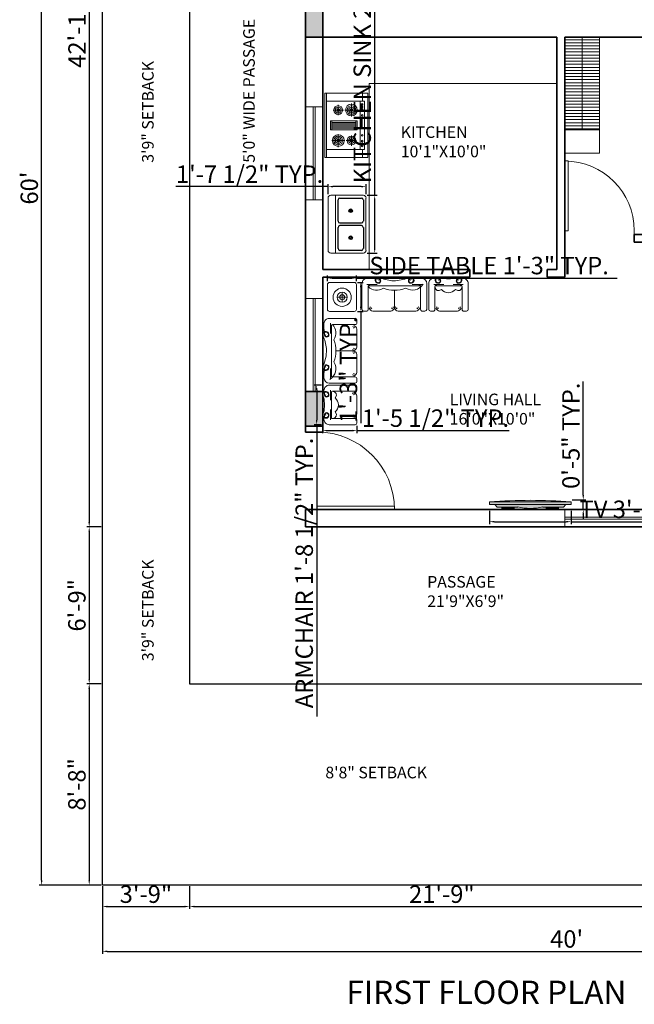
# Model space of a CAD drawing. Units: inches. Extents: x 3321 to 5237, y 11 to 1752.
# Tile 13 of 43: x 3979 to 4296, y 926 to 1434. Entities that reach past the tile are written whole.
import ezdxf

# ---------------------------------------------------------------- set-up
doc = ezdxf.new("R2010")
doc.units = ezdxf.units.IN
for name, color, linetype, lineweight in [('A-ANNO-DIMS', 2, 'Continuous', 18), ('A-ANNO-TEXT', 7, 'Continuous', 18), ('A-ANNO-TITL', 7, 'Continuous', 25), ('A-AREA-IDEN', 7, 'Continuous', 18), ('A-COLS', 1, 'Continuous', 35), ('A-DOOR', 4, 'Continuous', 18), ('A-EQPM', 8, 'Continuous', 18), ('A-FLOR-CASE', 8, 'Continuous', 18), ('A-FLOR-CASE-PATT', 8, 'Continuous', 13), ('A-FLOR-EDGE', 7, 'Continuous', 25), ('A-GLAZ', 5, 'Continuous', 18), ('A-WALL', 7, 'Continuous', 35), ('C-PROP', 7, 'Continuous', 30), ('FUR', 42, 'Continuous', 18), ('KITSHEN', 44, 'Continuous', 18), ('moveis', 254, 'Continuous', 5), ('parede', 7, 'Continuous', 30)]:
    doc.layers.add(name, color=color, linetype=linetype, lineweight=lineweight)
doc.layers.add('furn', color=17, linetype='Continuous')
doc.styles.get("Standard").update_dxf_attribs({"font": 'arial.ttf'})
doc.dimstyles.new('ISO-25', dxfattribs={"dimtxt": 9, "dimasz": 2.5, "dimexe": 1.25, "dimexo": 0.625, "dimtad": 1, "dimdec": 1, "dimlunit": 3, "dimtxsty": 'Standard', "dimcen": 2.5, "dimclrd": 4, "dimclre": 4, "dimclrt": 256, "dimadec": 0, "dimazin": 0, "dimtfac": 1, "dimtdec": 1, "dimtmove": 0, "dimatfit": 3, "dimfxl": 1, "dimarcsym": 0})

# ---------------------------------------------------------------- blocks, each defined once
blk = doc.blocks.new('*U2')
for p, q in [((0, 0), (0, -6)), ((-40, 0), (-40, -6))]:
    blk.add_line(p, q)
blk.add_lwpolyline([(0, 0), (0, 40), (-1.75, 40), (-1.75, 0)], close=True)
blk.add_arc((0, 0), 40, 90, 180)
blk = doc.blocks.new('*U4')
for p, q in [((0, 0), (0, -6)), ((-36, 0), (-36, -6))]:
    blk.add_line(p, q)
blk.add_lwpolyline([(0, 0), (0, 36), (-1.75, 36), (-1.75, 0)], close=True)
blk.add_arc((0, 0), 36, 90, 180)
blk = doc.blocks.new('*D53')
at = {"layer": 'A-ANNO-DIMS', "color": 0, "lineweight": -2, "transparency": 16777216}
for p, q in [((4020.76, 1687.34), (4013.34, 1687.34)), ((4014.59, 1684.84), (4014.59, 1174.84)), ((4020.76, 1172.34), (4013.34, 1172.34))]:
    blk.add_line(p, q, dxfattribs=at)
at = {"layer": 'A-ANNO-DIMS', "color": 0, "transparency": 16777216}
for points in [[(4014.17, 1684.84), (4015, 1684.84), (4014.59, 1687.34)], [(4014.17, 1174.84), (4015, 1174.84), (4014.59, 1172.34)]]:
    blk.add_solid(points, dxfattribs=at)
at = {"layer": 'Defpoints', "color": 0, "transparency": 16777216}
for p in [(4021.39, 1687.34), (4014.59, 1172.34), (4021.39, 1172.34)]:
    blk.add_point(p, dxfattribs=at)
at = {"layer": 'A-ANNO-DIMS', "color": 0, "transparency": 16777216, "insert": (4009.44, 1429.84), "char_height": 9, "attachment_point": 5, "rotation": 90}
blk.add_mtext('42\'-11"', dxfattribs=at)
blk = doc.blocks.new('*D54')
at = {"layer": 'A-ANNO-DIMS', "color": 0, "lineweight": -2, "transparency": 16777216}
for p, q in [((4020.76, 1172.34), (4013.34, 1172.34)), ((4014.59, 1169.84), (4014.59, 1093.84)), ((4020.76, 1091.34), (4013.34, 1091.34))]:
    blk.add_line(p, q, dxfattribs=at)
at = {"layer": 'A-ANNO-DIMS', "color": 0, "transparency": 16777216}
for points in [[(4014.17, 1169.84), (4015, 1169.84), (4014.59, 1172.34)], [(4014.17, 1093.84), (4015, 1093.84), (4014.59, 1091.34)]]:
    blk.add_solid(points, dxfattribs=at)
at = {"layer": 'Defpoints', "color": 0, "transparency": 16777216}
for p in [(4021.39, 1172.34), (4014.59, 1091.34), (4021.39, 1091.34)]:
    blk.add_point(p, dxfattribs=at)
at = {"layer": 'A-ANNO-DIMS', "color": 0, "transparency": 16777216, "insert": (4009.37, 1131.84), "char_height": 9, "attachment_point": 5, "rotation": 90}
blk.add_mtext('6\'-9"', dxfattribs=at)
blk = doc.blocks.new('*D55')
at = {"layer": 'A-ANNO-DIMS', "color": 0, "lineweight": -2, "transparency": 16777216}
for p, q in [((4020.76, 1091.34), (4013.34, 1091.34)), ((4014.59, 1088.84), (4014.59, 989.84)), ((4020.76, 987.34), (4013.34, 987.34))]:
    blk.add_line(p, q, dxfattribs=at)
at = {"layer": 'A-ANNO-DIMS', "color": 0, "transparency": 16777216}
for points in [[(4014.17, 1088.84), (4015, 1088.84), (4014.59, 1091.34)], [(4014.17, 989.84), (4015, 989.84), (4014.59, 987.34)]]:
    blk.add_solid(points, dxfattribs=at)
at = {"layer": 'Defpoints', "color": 0, "transparency": 16777216}
for p in [(4021.39, 1091.34), (4014.59, 987.34), (4021.39, 987.34)]:
    blk.add_point(p, dxfattribs=at)
at = {"layer": 'A-ANNO-DIMS', "color": 0, "transparency": 16777216, "insert": (4009.37, 1039.34), "char_height": 9, "attachment_point": 5, "rotation": 90}
blk.add_mtext('8\'-8"', dxfattribs=at)
blk = doc.blocks.new('*D56')
at = {"layer": 'A-ANNO-DIMS', "color": 0, "lineweight": -2, "transparency": 16777216}
for p, q in [((4021.39, 986.71), (4021.39, 974.99)), ((4066.39, 986.71), (4066.39, 974.99)), ((4023.89, 976.24), (4063.89, 976.24))]:
    blk.add_line(p, q, dxfattribs=at)
at = {"layer": 'A-ANNO-DIMS', "color": 0, "transparency": 16777216}
for points in [[(4023.89, 976.66), (4023.89, 975.82), (4021.39, 976.24)], [(4063.89, 976.66), (4063.89, 975.82), (4066.39, 976.24)]]:
    blk.add_solid(points, dxfattribs=at)
at = {"layer": 'Defpoints', "color": 0, "transparency": 16777216}
for p in [(4021.39, 987.34), (4066.39, 987.34), (4066.39, 976.24)]:
    blk.add_point(p, dxfattribs=at)
at = {"layer": 'A-ANNO-DIMS', "color": 0, "transparency": 16777216, "insert": (4043.89, 981.46), "char_height": 9, "attachment_point": 5}
blk.add_mtext('3\'-9"', dxfattribs=at)
blk = doc.blocks.new('*D57')
at = {"layer": 'A-ANNO-DIMS', "color": 0, "lineweight": -2, "transparency": 16777216}
for p, q in [((4066.39, 986.71), (4066.39, 974.99)), ((4327.39, 986.71), (4327.39, 974.99)), ((4068.89, 976.24), (4324.89, 976.24))]:
    blk.add_line(p, q, dxfattribs=at)
at = {"layer": 'A-ANNO-DIMS', "color": 0, "transparency": 16777216}
for points in [[(4068.89, 976.66), (4068.89, 975.82), (4066.39, 976.24)], [(4324.89, 976.66), (4324.89, 975.82), (4327.39, 976.24)]]:
    blk.add_solid(points, dxfattribs=at)
at = {"layer": 'Defpoints', "color": 0, "transparency": 16777216}
for p in [(4066.39, 987.34), (4327.39, 987.34), (4327.39, 976.24)]:
    blk.add_point(p, dxfattribs=at)
at = {"layer": 'A-ANNO-DIMS', "color": 0, "transparency": 16777216, "insert": (4196.89, 981.46), "char_height": 9, "attachment_point": 5}
blk.add_mtext('21\'-9"', dxfattribs=at)
blk = doc.blocks.new('*D65')
at = {"layer": 'A-ANNO-DIMS', "color": 0, "lineweight": -2, "transparency": 16777216}
for p, q in [((4020.76, 1707.34), (3988.74, 1707.34)), ((3989.99, 989.84), (3989.99, 1704.84)), ((4020.76, 987.34), (3988.74, 987.34))]:
    blk.add_line(p, q, dxfattribs=at)
at = {"layer": 'A-ANNO-DIMS', "color": 0, "transparency": 16777216}
for points in [[(3989.57, 1704.84), (3990.4, 1704.84), (3989.99, 1707.34)], [(3989.57, 989.84), (3990.4, 989.84), (3989.99, 987.34)]]:
    blk.add_solid(points, dxfattribs=at)
at = {"layer": 'Defpoints', "color": 0, "transparency": 16777216}
for p in [(3989.99, 1707.34), (4021.39, 1707.34), (4021.39, 987.34)]:
    blk.add_point(p, dxfattribs=at)
at = {"layer": 'A-ANNO-DIMS', "color": 0, "transparency": 16777216, "insert": (3984.77, 1347.34), "char_height": 9, "attachment_point": 5, "rotation": 90}
blk.add_mtext("60'", dxfattribs=at)
blk = doc.blocks.new('*D66')
at = {"layer": 'A-ANNO-DIMS', "color": 0, "lineweight": -2, "transparency": 16777216}
for p, q in [((4021.39, 986.71), (4021.39, 951.84)), ((4501.39, 986.71), (4501.39, 951.84)), ((4023.89, 953.09), (4498.89, 953.09))]:
    blk.add_line(p, q, dxfattribs=at)
at = {"layer": 'A-ANNO-DIMS', "color": 0, "transparency": 16777216}
for points in [[(4023.89, 953.51), (4023.89, 952.68), (4021.39, 953.09)], [(4498.89, 953.51), (4498.89, 952.68), (4501.39, 953.09)]]:
    blk.add_solid(points, dxfattribs=at)
at = {"layer": 'Defpoints', "color": 0, "transparency": 16777216}
for p in [(4021.39, 987.34), (4501.39, 987.34), (4501.39, 953.09)]:
    blk.add_point(p, dxfattribs=at)
at = {"layer": 'A-ANNO-DIMS', "color": 0, "transparency": 16777216, "insert": (4261.39, 958.31), "char_height": 9, "attachment_point": 5}
blk.add_mtext("40'", dxfattribs=at)
blk = doc.blocks.new('Oven Pln 001')
at = {"layer": 'KITSHEN'}
for p, q in [((2216.8, 1000.7), (2306.8, 1000.7)), ((2216.8, 942.7), (2216.8, 1000.7)), ((2228.1, 996.2), (2295.5, 996.2)), ((2228.1, 942.7), (2228.1, 996.2)), ((2295.5, 996.2), (2295.5, 942.7)), ((2306.8, 942.7), (2306.8, 1000.7)), ((2228.1, 993.2), (2216.8, 993.2)), ((2228.1, 990.1), (2295.5, 990.1)), ((2240.4, 968.6), (2240.4, 987)), ((2255.6, 984), (2267.9, 984)), ((2257.7, 950.3), (2257.7, 984)), ((2259.7, 984), (2259.7, 950.3)), ((2261.8, 950.3), (2261.8, 984)), ((2263.8, 984), (2263.8, 950.3)), ((2265.9, 950.3), (2265.9, 984)), ((2283.2, 970.6), (2283.2, 985)), ((2295.5, 993.2), (2306.8, 993.2)), ((2231.2, 977.8), (2249.6, 977.8)), ((2240.4, 952.2), (2240.4, 966.6)), ((2276, 977.8), (2290.4, 977.8)), ((2283.2, 950.2), (2283.2, 968.6)), ((2233.2, 959.4), (2247.6, 959.4)), ((2274, 959.4), (2292.4, 959.4)), ((2216.8, 940.7), (2216.8, 942.7)), ((2306.8, 942.7), (2216.8, 942.7)), ((2306.8, 940.7), (2216.8, 940.7)), ((2267.9, 950.3), (2255.6, 950.3)), ((2306.8, 940.7), (2306.8, 942.7))]:
    blk.add_line(p, q, dxfattribs=at)
blk.add_lwpolyline([(2255.6, 948.3), (2255.6, 986), (2267.9, 986), (2267.9, 948.3)], close=True, dxfattribs=at)
for centre, radius in [((2232.6, 992.9), 1.16), ((2236.1, 992.9), 1.16), ((2239.7, 992.9), 1.16), ((2247.7, 992.9), 1.16), ((2275.9, 992.9), 1.16), ((2283.9, 992.9), 1.16), ((2287.5, 992.9), 1.16), ((2290.9, 992.9), 1.16), ((2240.4, 977.8), 8.19), ((2240.4, 977.8), 6.14), ((2240.4, 977.8), 4.09), ((2240.4, 977.8), 2.05), ((2283.2, 977.8), 6.14), ((2283.2, 977.8), 4.09), ((2283.2, 977.8), 2.05), ((2283.2, 959.4), 8.19), ((2240.4, 959.4), 6.14), ((2240.4, 959.4), 4.09), ((2240.4, 959.4), 2.05), ((2283.2, 959.4), 6.14), ((2283.2, 959.4), 4.09), ((2283.2, 959.4), 2.05)]:
    blk.add_circle(centre, radius, dxfattribs=at)
blk = doc.blocks.new('ps sin 19')
at = {"layer": 'furn'}
for p, q in [((5312.3, 277.7), (5312.3, 306.3)), ((5314.6, 308.7), (5342.6, 308.7)), ((5345, 277.7), (5345, 306.3)), ((5348.6, 306.3), (5348.6, 277.7)), ((5350.9, 308.7), (5378.9, 308.7)), ((5381.3, 306.3), (5381.3, 277.7)), ((5342.6, 275.3), (5314.6, 275.3)), ((5378.9, 275.3), (5350.9, 275.3))]:
    blk.add_line(p, q, dxfattribs=at)
for centre, radius in [((5328.9, 292), 2.38), ((5328.9, 292), 1.19), ((5364.6, 292), 2.38), ((5364.6, 292), 1.19)]:
    blk.add_circle(centre, radius, dxfattribs=at)
for centre, start, end in [((5314.6, 306.3), 90, 180), ((5342.6, 306.3), 0, 90), ((5350.9, 306.3), 90, 180), ((5378.9, 306.3), 0, 90), ((5314.6, 277.7), 180, 270), ((5342.6, 277.7), 270, 0), ((5350.9, 277.7), 180, 270), ((5378.9, 277.7), 270, 0)]:
    blk.add_arc(centre, 2.38, start, end, dxfattribs=at)
at = {"layer": 'KITSHEN'}
for p, q in [((5308.7, 275.3), (5308.7, 318.2)), ((5308.7, 312.2), (5384.9, 312.2)), ((5312.3, 321.8), (5381.3, 321.8)), ((5384.9, 318.2), (5384.9, 275.3)), ((5381.3, 271.8), (5312.3, 271.8))]:
    blk.add_line(p, q, dxfattribs=at)
for centre, start, end in [((5312.3, 318.2), 90, 180), ((5381.3, 318.2), 0, 90), ((5312.3, 275.3), 180, 270), ((5381.3, 275.3), 270, 0)]:
    blk.add_arc(centre, 3.57, start, end, dxfattribs=at)
blk = doc.blocks.new('sofa-34')
at = {"color": 0, "linetype": 'ByBlock'}
for p, q in [((-0.15, 0.15), (-0.15, 0.874)), ((-0.026, 0.924), (-0.1, 0.924)), ((0.024, 0.236), (0.024, 0.874)), ((0.05, 0.838), (0.05, 0.838)), ((0.101, 0.857), (0.126, 0.829)), ((0.657, 0.925), (0.153, 0.925)), ((0.71, 0.857), (0.684, 0.829)), ((0.76, 0.838), (0.76, 0.838)), ((0.76, 0.838), (0.76, 0.838)), ((0.786, 0.236), (0.786, 0.874)), ((0.836, 0.924), (0.91, 0.924)), ((0.96, 0.15), (0.96, 0.874)), ((0.09, 0.806), (0.068, 0.824)), ((0.72, 0.806), (0.742, 0.824)), ((-0.01, 0.18), (0.274, 0.18)), ((0.029, 0.214), (0.781, 0.214)), ((0.82, 0.18), (0.536, 0.18))]:
    blk.add_line(p, q, dxfattribs=at)
blk.add_arc((0.405, 0.148), 0.258, 40.7983, 139.2017, dxfattribs=at)
at = {"color": 0, "linetype": 'ByBlock', "extrusion": (0, 0, -1)}
for centre, major_axis, ratio, start_param, end_param in [((-0.1, 0.874), (0.0354, 0.0354), 1, 3.926992, 5.497787), ((-0.026, 0.874), (-0.0354, 0.0354), 1, 0.785398, 2.356196), ((0.2, 0.766), (0.117, 0.117), 1, 4.372209, 5.213218), ((0.61, 0.766), (0.117, 0.117), 1, -0.500829, 0.34018), ((0.5, -0.587), (-0.415, 0.931), 0.264583, -0.381915, 0.387685), ((0, 0.15), (0.106, 0.106), 1, 2.356194, 3.926992), ((0.179, -0.658), (-0.251, 0.635), 0.885019, 0.124301, 0.339591), ((0.117, 0.052), (-0.0624, 0.0624), 1, 4.675944, 7.152385), ((0.074, 0.236), (-0.0354, 0.0354), 1, 3.926991, 5.497788), ((0.13, 0.052), (-0.059, 0.059), 1, 3.186406, 6.094039), ((0.114, 0.063), (-0.0458, 0.0458), 1, 6.094039, 8.043134), ((0.129, 0.073), (-0.0414, 0.0414), 1, 2.230507, 4.423483), ((0.139, 0.08), (0.0245, 0.0245), 1, 0.189152, 2.952444), ((0.118, 0.071), (0.0491, 0.0491), 1, -0.701597, 0.659711), ((0.352, -0.558), (0.735, 0.107), 0.76838, 4.597815, 5.20076)]:
    blk.add_ellipse(centre, major_axis=major_axis, ratio=ratio, start_param=start_param, end_param=end_param, dxfattribs=at)
at = {"color": 0, "linetype": 'ByBlock'}
for centre, major_axis, ratio, start_param, end_param in [((0.836, 0.874), (0.0354, 0.0354), 1, 0.785398, 2.356196), ((0.91, 0.874), (-0.0354, 0.0354), 1, 3.926992, 5.497787), ((0.31, -0.587), (0.415, 0.931), 0.264583, -0.381915, 0.387685), ((0.681, 0.073), (0.0414, 0.0414), 1, 2.230507, 4.423483), ((0.692, 0.071), (-0.0491, 0.0491), 1, -0.701597, 0.659711), ((0.68, 0.052), (0.059, 0.059), 1, 3.186406, 6.094039), ((0.671, 0.08), (-0.0245, 0.0245), 1, 0.189152, 2.952444), ((0.696, 0.063), (0.0458, 0.0458), 1, 6.094039, 8.043134), ((0.631, -0.658), (0.251, 0.635), 0.885019, 0.124301, 0.339591), ((0.693, 0.052), (0.0624, 0.0624), 1, 4.675944, 7.152385), ((0.736, 0.236), (0.0354, 0.0354), 1, 3.926991, 5.497788), ((0.81, 0.15), (-0.106, 0.106), 1, 2.356194, 3.926992)]:
    blk.add_ellipse(centre, major_axis=major_axis, ratio=ratio, start_param=start_param, end_param=end_param, dxfattribs=at)
blk = doc.blocks.new('sofa-33')
at = {"color": 0, "linetype": 'ByBlock'}
for p, q in [((-0.15, 0.15), (-0.15, 0.874)), ((-0.026, 0.924), (-0.1, 0.924)), ((0.024, 0.236), (0.024, 0.874)), ((0.05, 0.838), (0.05, 0.838)), ((0.101, 0.857), (0.126, 0.829)), ((0.657, 0.925), (0.153, 0.925)), ((0.71, 0.857), (0.684, 0.829)), ((0.76, 0.838), (0.76, 0.336)), ((0.76, 0.838), (0.76, 0.838)), ((0.76, 0.838), (0.76, 0.838)), ((0.811, 0.857), (0.837, 0.829)), ((0.863, 0.925), (1.367, 0.925)), ((1.42, 0.857), (1.394, 0.829)), ((1.47, 0.838), (1.47, 0.838)), ((1.47, 0.838), (1.47, 0.838)), ((1.496, 0.236), (1.496, 0.874)), ((1.62, 0.924), (1.546, 0.924)), ((1.67, 0.15), (1.67, 0.874)), ((0.09, 0.806), (0.068, 0.824)), ((0.72, 0.806), (0.742, 0.824)), ((0.8, 0.806), (0.778, 0.824)), ((1.43, 0.806), (1.452, 0.824)), ((-0.01, 0.18), (0.274, 0.18)), ((0, 0), (0.136, 0)), ((0.029, 0.214), (1.491, 0.214)), ((1.542, 0.18), (1.258, 0.18)), ((1.532, 0), (1.397, 0))]:
    blk.add_line(p, q, dxfattribs=at)
at = {"color": 0, "linetype": 'ByBlock', "extrusion": (0, 0, -1)}
for centre, major_axis, ratio, start_param, end_param in [((-0.1, 0.874), (0.0354, 0.0354), 1, 3.926992, 5.497787), ((-0.026, 0.874), (-0.0354, 0.0354), 1, 0.785398, 2.356196), ((0.2, 0.766), (0.117, 0.117), 1, 4.372209, 5.213218), ((0.61, 0.766), (0.117, 0.117), 1, -0.500829, 0.34018), ((0.91, 0.766), (0.117, 0.117), 1, 4.372209, 5.213218), ((1.321, 0.766), (-0.117, 0.117), 1, 1.069968, 1.910976), ((1.546, 0.874), (-0.0354, 0.0354), 1, 5.497786, 7.068583), ((1.62, 0.874), (0.0354, 0.0354), 1, -0.785398, 0.785398), ((0.323, -0.666), (-0.093, 1), 0.551284, -0.397889, 0.397889), ((0.766, -0.668), (-0.003, 1.004), 0.922365, -0.343589, 0.343589), ((1.147, -0.534), (0.2, 0.861), 0.59532, -0.502747, 0.502747), ((0, 0.15), (0.106, 0.106), 1, 2.356194, 3.926992), ((0.074, 0.236), (-0.0354, 0.0354), 1, 3.926991, 5.497788), ((0.282, -0.661), (-0.479, 0.479), 1, 0.566947, 0.842011), ((0.308, 0.052), (-0.0624, 0.0624), 1, 4.675944, 7.152385), ((0.321, 0.052), (-0.059, 0.059), 1, 3.186406, 6.094039), ((0.305, 0.063), (-0.0458, 0.0458), 1, 6.094039, 8.043134), ((0.32, 0.073), (-0.0414, 0.0414), 1, 2.230507, 4.423483), ((0.33, 0.08), (0.0245, 0.0245), 1, 0.189152, 2.952444), ((0.309, 0.071), (0.0491, 0.0491), 1, -0.701597, 0.659711), ((0.878, -1.382), (-0.323, 1.429), 0.878591, -0.144977, 0.144977), ((0.667, -1.39), (1.036, 1.036), 1, 5.547613, 5.837566), ((1.212, 0.073), (-0.0414, 0.0414), 1, 3.430501, 5.623477), ((1.223, 0.071), (-0.0491, 0.0491), 1, 5.623477, 6.984784), ((1.211, 0.052), (0.059, 0.059), 1, 0.189149, 3.096782), ((1.202, 0.08), (0.0245, 0.0245), 1, 1.759947, 4.52324), ((1.227, 0.063), (0.0458, 0.0458), 1, 4.52324, 6.472335), ((1.25, -0.661), (0.479, 0.479), 1, 5.441177, 5.716241), ((1.225, 0.052), (-0.0624, 0.0624), 1, 0.701599, 3.17804), ((1.446, 0.236), (0.0354, 0.0354), 1, 0.785397, 2.356194), ((1.52, 0.15), (0.106, 0.106), 1, 0.785398, 2.356194)]:
    blk.add_ellipse(centre, major_axis=major_axis, ratio=ratio, start_param=start_param, end_param=end_param, dxfattribs=at)
blk = doc.blocks.new('table-31')
at = {"color": 0, "linetype": 'ByBlock'}
for p, q in [((-0.203, 0.167), (-0.203, -0.176)), ((0.168, 0.195), (-0.175, 0.195)), ((0.197, 0.167), (0.197, -0.176)), ((-0.069, 0), (0.069, 0)), ((0, -0.069), (0, 0.069)), ((0.168, -0.205), (-0.175, -0.205))]:
    blk.add_line(p, q, dxfattribs=at)
for radius in [0.126, 0.0689, 0.0353]:
    blk.add_circle((0, 0), radius, dxfattribs=at)
for centre, start, end in [((-0.175, 0.167), 90, 180), ((0.168, 0.167), 0, 90), ((-0.175, -0.176), 180, 270), ((0.168, -0.176), 270, 0)]:
    blk.add_arc(centre, 0.0286, start, end, dxfattribs=at)
blk = doc.blocks.new('PLASMA 2')
at = {"layer": 'moveis', "ltscale": 0.08}
h = blk.add_hatch(dxfattribs=at)
h.set_pattern_fill('_USER,_O', color=256, scale=0.008, double=1, pattern_type=0)
h.set_pattern_definition([(360, (-4.134502, -6.848382), (0, 0.008), []), (90, (-4.134502, -6.848382), (-0.008, 0), [])])
h.paths.add_polyline_path([(-0.21, -0.097), (-0.362, -0.097), (-0.362, -0.111), (-0.21, -0.111)])
h = blk.add_hatch(dxfattribs=at)
h.set_pattern_fill('_USER,_O', color=256, scale=0.008, double=1, pattern_type=0)
h.set_pattern_definition([(180, (4.134502, -6.848382), (0, 0.008), []), (90, (4.134502, -6.848382), (0.008, 0), [])])
h.paths.add_polyline_path([(0.21, -0.097), (0.362, -0.097), (0.362, -0.111), (0.21, -0.111)])
at = {"layer": 'parede', "ltscale": 0.08}
h = blk.add_hatch(color=256, dxfattribs=at)
h.dxf.hatch_style = 1
h.set_gradient(color1=(131, 136, 145), one_color=1, tint=1, name='CURVED')
h.paths.add_polyline_path([(-0.535, -0.022), (0.535, -0.022, 0.040195)])
h = blk.add_hatch(color=256, dxfattribs=at)
h.dxf.hatch_style = 1
h.set_gradient(color1=(131, 136, 145), color2=(0, 0, 0), one_color=1, name='CURVED')
h.paths.add_polyline_path([(0.535, -0.022), (-0.535, -0.022), (-0.535, -0.055), (0.535, -0.055)])
h = blk.add_hatch(color=256, dxfattribs=at)
h.dxf.hatch_style = 1
h.set_gradient(color1=(131, 136, 145), one_color=1, tint=1, name='CYLINDER')
h.paths.add_polyline_path([(0.467, -0.055), (-0.467, -0.055), (-0.436, -0.088), (-0.164, -0.088, 0.114423), (0.164, -0.088), (0.436, -0.088)])
h = blk.add_hatch(color=256, dxfattribs=at)
h.dxf.hatch_style = 1
h.set_gradient(color1=(131, 136, 145), color2=(0, 0, 0), one_color=1, name='CURVED')
h.paths.add_polyline_path([(0.372, -0.088), (0.164, -0.088, -0.114423), (-0.164, -0.088), (-0.372, -0.088), (-0.372, -0.12), (0.372, -0.12)])
h.paths.add_polyline_path([(-0.21, -0.111), (-0.362, -0.111), (-0.362, -0.097), (-0.21, -0.097)], flags=16)
h.paths.add_polyline_path([(0.21, -0.111), (0.21, -0.097), (0.362, -0.097), (0.362, -0.111)], flags=16)
at = {"layer": 'moveis', "ltscale": 0.08}
for p, q in [((-0.535, -0.022), (-0.535, -0.055)), ((-0.535, -0.022), (0.535, -0.022)), ((0.535, -0.055), (-0.535, -0.055)), ((-0.467, -0.055), (-0.436, -0.088)), ((-0.436, -0.088), (-0.164, -0.088)), ((-0.372, -0.088), (-0.372, -0.12)), ((-0.372, -0.12), (0.372, -0.12)), ((0.164, -0.088), (0.436, -0.088)), ((0.372, -0.088), (0.372, -0.12)), ((0.467, -0.055), (0.436, -0.088)), ((0.535, -0.055), (0.535, -0.022))]:
    blk.add_line(p, q, dxfattribs=at)
for points in [[(-0.362, -0.097), (-0.21, -0.097), (-0.21, -0.111), (-0.362, -0.111)], [(0.362, -0.097), (0.21, -0.097), (0.21, -0.111), (0.362, -0.111)]]:
    blk.add_lwpolyline(points, close=True, dxfattribs=at)
for centre, radius, start, end in [((0, -6.666), 6.666, 85.3965, 94.6035), ((0, 0.618), 0.724, 256.9449, 283.0551)]:
    blk.add_arc(centre, radius, start, end, dxfattribs=at)
blk = doc.blocks.new('COL-9X18-IN')
h = blk.add_hatch(color=256)
h.dxf.hatch_style = 1
h.paths.add_polyline_path([(9, 18), (0, 18), (0, 0), (9, 0)])
blk.add_lwpolyline([(0, 0), (9, 0), (9, 18), (0, 18)], close=True)
blk = doc.blocks.new('WIN-48IN-9IN-WALL')
for p, q in [((0, 0), (0, 9)), ((48, 0), (48, 9)), ((0, 5), (48, 5)), ((0, 4), (48, 4))]:
    blk.add_line(p, q)
blk = doc.blocks.new('PROPERTY-40X60FT')
for p, q in [((0, 720), (480, 720)), ((480, 720), (480, 0))]:
    blk.add_line(p, q)
blk = doc.blocks.new('*D205')
at = {"layer": 'A-ANNO-DIMS', "color": 4, "lineweight": -2, "transparency": 16777216}
for p, q in [((4134.6, 1245.56), (4130.92, 1245.56)), ((4132.17, 1243.06), (4132.17, 1227.63)), ((4134.6, 1225.13), (4130.92, 1225.13)), ((4132.17, 1225.13), (4132.17, 1074.48))]:
    blk.add_line(p, q, dxfattribs=at)
at = {"layer": 'A-ANNO-DIMS', "color": 4, "transparency": 16777216}
for points in [[(4131.75, 1243.06), (4132.58, 1243.06), (4132.17, 1245.56)], [(4131.75, 1227.63), (4132.58, 1227.63), (4132.17, 1225.13)]]:
    blk.add_solid(points, dxfattribs=at)
at = {"layer": 'Defpoints', "color": 0, "transparency": 16777216}
for p in [(4135.23, 1245.56), (4132.17, 1225.13), (4135.23, 1225.13)]:
    blk.add_point(p, dxfattribs=at)
at = {"layer": 'A-ANNO-DIMS', "transparency": 16777216, "insert": (4126.89, 1148.55), "char_height": 9, "attachment_point": 5, "rotation": 90}
blk.add_mtext('ARMCHAIR 1\'-8 1/2" TYP.', dxfattribs=at)
blk = doc.blocks.new('*D206')
at = {"layer": 'A-ANNO-DIMS', "color": 4, "lineweight": -2, "transparency": 16777216}
for p, q in [((4135.23, 1224.5), (4135.23, 1220.81)), ((4137.73, 1222.06), (4150.47, 1222.06)), ((4152.97, 1224.5), (4152.97, 1220.81)), ((4152.97, 1222.06), (4231.7, 1222.06))]:
    blk.add_line(p, q, dxfattribs=at)
at = {"layer": 'A-ANNO-DIMS', "color": 4, "transparency": 16777216}
for points in [[(4137.73, 1222.48), (4137.73, 1221.65), (4135.23, 1222.06)], [(4150.47, 1222.48), (4150.47, 1221.65), (4152.97, 1222.06)]]:
    blk.add_solid(points, dxfattribs=at)
at = {"layer": 'Defpoints', "color": 0, "transparency": 16777216}
for p in [(4135.23, 1225.13), (4152.97, 1225.13), (4152.97, 1222.06)]:
    blk.add_point(p, dxfattribs=at)
at = {"layer": 'A-ANNO-DIMS', "transparency": 16777216, "insert": (4193.58, 1227.34), "char_height": 9, "attachment_point": 5}
blk.add_mtext('1\'-5 1/2" TYP.', dxfattribs=at)
blk = doc.blocks.new('*D213')
at = {"layer": 'A-ANNO-DIMS', "color": 4, "lineweight": -2, "transparency": 16777216}
for p, q in [((4137.74, 1299.24), (4137.74, 1302.11)), ((4152.71, 1299.24), (4152.71, 1302.11)), ((4140.24, 1300.86), (4150.21, 1300.86)), ((4152.71, 1300.86), (4287.44, 1300.86))]:
    blk.add_line(p, q, dxfattribs=at)
at = {"layer": 'A-ANNO-DIMS', "color": 4, "transparency": 16777216}
for points in [[(4140.24, 1301.27), (4140.24, 1300.44), (4137.74, 1300.86)], [(4150.21, 1301.27), (4150.21, 1300.44), (4152.71, 1300.86)]]:
    blk.add_solid(points, dxfattribs=at)
at = {"layer": 'Defpoints', "color": 0, "transparency": 16777216}
for p in [(4137.74, 1298.61), (4152.71, 1300.86), (4152.71, 1298.61)]:
    blk.add_point(p, dxfattribs=at)
at = {"layer": 'A-ANNO-DIMS', "transparency": 16777216, "insert": (4221.32, 1306.14), "char_height": 9, "attachment_point": 5}
blk.add_mtext('SIDE TABLE 1\'-3" TYP.', dxfattribs=at)
blk = doc.blocks.new('*D214')
at = {"layer": 'A-ANNO-DIMS', "color": 4, "lineweight": -2, "transparency": 16777216}
for p, q in [((4153.33, 1298.61), (4156.2, 1298.61)), ((4154.95, 1296.11), (4154.95, 1286.14)), ((4153.33, 1283.64), (4156.2, 1283.64)), ((4154.95, 1283.64), (4154.95, 1225.88))]:
    blk.add_line(p, q, dxfattribs=at)
at = {"layer": 'A-ANNO-DIMS', "color": 4, "transparency": 16777216}
for points in [[(4154.53, 1296.11), (4155.37, 1296.11), (4154.95, 1298.61)], [(4154.53, 1286.14), (4155.37, 1286.14), (4154.95, 1283.64)]]:
    blk.add_solid(points, dxfattribs=at)
at = {"layer": 'Defpoints', "color": 0, "transparency": 16777216}
for p in [(4152.71, 1298.61), (4152.71, 1283.64), (4154.95, 1283.64)]:
    blk.add_point(p, dxfattribs=at)
at = {"layer": 'A-ANNO-DIMS', "transparency": 16777216, "insert": (4149.73, 1253.51), "char_height": 9, "attachment_point": 5, "rotation": 90}
blk.add_mtext('1\'-3" TYP.', dxfattribs=at)
blk = doc.blocks.new('*D215')
at = {"layer": 'A-ANNO-DIMS', "color": 4, "lineweight": -2, "transparency": 16777216}
for p, q in [((4221.54, 1180.71), (4221.54, 1173.77)), ((4263.67, 1180.71), (4263.67, 1173.77)), ((4224.04, 1175.02), (4261.17, 1175.02)), ((4263.67, 1175.02), (4342.06, 1175.02))]:
    blk.add_line(p, q, dxfattribs=at)
at = {"layer": 'A-ANNO-DIMS', "color": 4, "transparency": 16777216}
for points in [[(4224.04, 1175.44), (4224.04, 1174.6), (4221.54, 1175.02)], [(4261.17, 1175.44), (4261.17, 1174.6), (4263.67, 1175.02)]]:
    blk.add_solid(points, dxfattribs=at)
at = {"layer": 'Defpoints', "color": 0, "transparency": 16777216}
for p in [(4221.54, 1181.34), (4263.67, 1181.34), (4263.67, 1175.02)]:
    blk.add_point(p, dxfattribs=at)
at = {"layer": 'A-ANNO-DIMS', "transparency": 16777216, "insert": (4304.12, 1180.24), "char_height": 9, "attachment_point": 5}
blk.add_mtext('TV 3\'-6" TYP.', dxfattribs=at)
blk = doc.blocks.new('*D216')
at = {"layer": 'A-ANNO-DIMS', "color": 4, "lineweight": -2, "transparency": 16777216}
for p, q in [((4269.99, 1188.85), (4269.99, 1247.45)), ((4264.29, 1186.35), (4271.24, 1186.35)), ((4269.99, 1181.34), (4269.99, 1186.35)), ((4264.29, 1181.34), (4271.24, 1181.34)), ((4269.99, 1178.84), (4269.99, 1176.34))]:
    blk.add_line(p, q, dxfattribs=at)
at = {"layer": 'A-ANNO-DIMS', "color": 4, "transparency": 16777216}
for points in [[(4269.57, 1188.85), (4270.4, 1188.85), (4269.99, 1186.35)], [(4269.57, 1178.84), (4270.4, 1178.84), (4269.99, 1181.34)]]:
    blk.add_solid(points, dxfattribs=at)
at = {"layer": 'Defpoints', "color": 0, "transparency": 16777216}
for p in [(4263.67, 1186.35), (4269.99, 1186.35), (4263.67, 1181.34)]:
    blk.add_point(p, dxfattribs=at)
at = {"layer": 'A-ANNO-DIMS', "transparency": 16777216, "insert": (4264.77, 1219.4), "char_height": 9, "attachment_point": 5, "rotation": 90}
blk.add_mtext('0\'-5" TYP.', dxfattribs=at)
blk = doc.blocks.new('*D219')
at = {"layer": 'A-ANNO-DIMS', "color": 4, "lineweight": -2, "transparency": 16777216}
for p, q in [((4162.16, 1343.6), (4162.16, 1493.33)), ((4158.31, 1343.6), (4163.41, 1343.6)), ((4162.16, 1316.25), (4162.16, 1341.1)), ((4158.31, 1313.75), (4163.41, 1313.75))]:
    blk.add_line(p, q, dxfattribs=at)
at = {"layer": 'A-ANNO-DIMS', "color": 4, "transparency": 16777216}
for points in [[(4161.74, 1341.1), (4162.58, 1341.1), (4162.16, 1343.6)], [(4161.74, 1316.25), (4162.58, 1316.25), (4162.16, 1313.75)]]:
    blk.add_solid(points, dxfattribs=at)
at = {"layer": 'Defpoints', "color": 0, "transparency": 16777216}
for p in [(4157.68, 1343.6), (4162.16, 1343.6), (4157.68, 1313.75)]:
    blk.add_point(p, dxfattribs=at)
at = {"layer": 'A-ANNO-DIMS', "transparency": 16777216, "insert": (4156.88, 1419.72), "char_height": 9, "attachment_point": 5, "rotation": 90}
blk.add_mtext('KITCHEN SINK 2\'-6" TYP.', dxfattribs=at)
blk = doc.blocks.new('*D220')
at = {"layer": 'A-ANNO-DIMS', "color": 4, "lineweight": -2, "transparency": 16777216}
for p, q in [((4138.09, 1348.08), (4059.36, 1348.08)), ((4138.09, 1344.23), (4138.09, 1349.33)), ((4155.18, 1348.08), (4140.59, 1348.08)), ((4157.68, 1344.23), (4157.68, 1349.33))]:
    blk.add_line(p, q, dxfattribs=at)
at = {"layer": 'A-ANNO-DIMS', "color": 4, "transparency": 16777216}
for points in [[(4140.59, 1348.5), (4140.59, 1347.67), (4138.09, 1348.08)], [(4155.18, 1348.5), (4155.18, 1347.67), (4157.68, 1348.08)]]:
    blk.add_solid(points, dxfattribs=at)
at = {"layer": 'Defpoints', "color": 0, "transparency": 16777216}
for p in [(4138.09, 1348.08), (4138.09, 1343.6), (4157.68, 1343.6)]:
    blk.add_point(p, dxfattribs=at)
at = {"layer": 'A-ANNO-DIMS', "transparency": 16777216, "insert": (4097.48, 1353.36), "char_height": 9, "attachment_point": 5}
blk.add_mtext('1\'-7 1/2" TYP.', dxfattribs=at)

msp = doc.modelspace()

# ---------------------------------------------------------------- hatches: boundary and pattern name
at = {"layer": 'A-FLOR-CASE-PATT'}
h = msp.add_hatch(dxfattribs=at)
h.set_pattern_fill('ANSI31', color=256, scale=0.5, angle=135)
h.set_pattern_definition([(180, (-735.7874, -1e-13), (-1e-16, -1.5875), [])])
h.paths.add_polyline_path([(4260.39, 1377.34), (4278.39, 1377.34), (4278.39, 1425.34), (4260.39, 1425.34)])

# ---------------------------------------------------------------- linework, layer by layer
at = {"layer": 'A-FLOR-CASE'}
for p, q in [((4269.39, 1377.34), (4269.39, 1425.34)), ((4278.39, 1425.34), (4278.39, 1365.34)), ((4159.39, 1401.34), (4159.39, 1305.34)), ((4159.39, 1401.34), (4256.39, 1401.34)), ((4260.39, 1377.34), (4278.39, 1377.34)), ((4260.39, 1365.34), (4278.39, 1365.34))]:
    msp.add_line(p, q, dxfattribs=at)
at = {"layer": 'A-FLOR-EDGE'}
for p, q in [((4066.39, 1687.34), (4066.39, 1091.34)), ((4066.39, 1091.34), (4465.39, 1091.34))]:
    msp.add_line(p, q, dxfattribs=at)
at = {"layer": 'A-WALL'}
for p, q in [((4126.39, 1443.34), (4126.39, 1221.34)), ((4135.39, 1425.34), (4135.39, 1305.34)), ((4135.39, 1425.34), (4256.39, 1425.34)), ((4256.39, 1425.34), (4256.39, 1305.34)), ((4260.39, 1425.34), (4260.39, 1301.34)), ((4260.39, 1425.34), (4327.39, 1425.34)), ((4296.39, 1323.34), (4392.39, 1323.34)), ((4296.39, 1323.34), (4296.39, 1319.34)), ((4296.39, 1319.34), (4392.39, 1319.34)), ((4135.39, 1305.34), (4211.39, 1305.34)), ((4211.39, 1305.34), (4211.39, 1301.34)), ((4251.39, 1305.34), (4251.39, 1301.34)), ((4251.39, 1305.34), (4256.39, 1305.34)), ((4135.39, 1301.34), (4211.39, 1301.34)), ((4135.39, 1301.34), (4135.39, 1221.34)), ((4251.39, 1301.34), (4260.39, 1301.34)), ((4126.39, 1221.34), (4135.39, 1221.34)), ((4126.39, 1181.34), (4327.39, 1181.34)), ((4126.39, 1181.34), (4126.39, 1172.34)), ((4126.39, 1172.34), (4456.39, 1172.34))]:
    msp.add_line(p, q, dxfattribs=at)

# ---------------------------------------------------------------- block references
at = {"layer": 'A-COLS', "rotation": 180}
for p in [(4135.39, 1443.34), (4135.39, 1242.34)]:
    msp.add_blockref('COL-9X18-IN', p, dxfattribs=at)
at = {"layer": 'A-DOOR', "xscale": -1}
msp.add_blockref('*U4', (4260.39, 1325.34), dxfattribs=at)
at = {"layer": 'A-DOOR', "rotation": 270}
msp.add_blockref('*U2', (4132.39, 1181.34), dxfattribs=at)
at = {"layer": 'A-EQPM', "xscale": 39.3701, "yscale": 39.3701, "zscale": 39.3701}
msp.add_blockref('PLASMA 2', (4242.61, 1186.06), dxfattribs=at)
at = {"layer": 'A-GLAZ'}
for p, rotation in [((4135.39, 1341.34), 89.99999999999613), ((4135.39, 1242.34), 89.99999999999802)]:
    msp.add_blockref('WIN-48IN-9IN-WALL', p, dxfattribs=dict(at, rotation=rotation))
msp.add_blockref('WIN-48IN-9IN-WALL', (4260.39, 1172.34), dxfattribs=at)
at = {"layer": 'C-PROP', "rotation": 180}
msp.add_blockref('PROPERTY-40X60FT', (4501.39, 1707.34), dxfattribs=at)
at = {"layer": 'FUR'}
for name, p, xscale, yscale, zscale, rotation in [('table-31', (4145.34, 1290.95), -37.41559934897337, 37.41559934897337, 37.41559934897337, 180), ('sofa-33', (4158.35, 1300.77), -18.40353949668526, 18.40353949668526, 18.40353949668526, 180), ('sofa-34', (4192.85, 1300.78), -18.40353949668526, 18.40353949668526, 18.40353949668526, 180), ('sofa-33', (4135.95, 1277.3), 18.40353949668526, 18.40353949668526, 18.40353949668526, 270), ('sofa-34', (4135.94, 1242.8), 18.40353949668526, 18.40353949668526, 18.40353949668526, 270)]:
    msp.add_blockref(name, p, dxfattribs=dict(at, xscale=xscale, yscale=yscale, zscale=zscale, rotation=rotation))
at = {"layer": 'KITSHEN'}
for name, p, xscale, yscale, zscale, rotation in [('Oven Pln 001', (3789.74, 2213.39), 0.3685700214197002, 0.3685700214197002, 0.3685700214197002, 270), ('ps sin 19', (4264.15, -766.07), 0.3917772908061623, 0.3917772908061623, 0.3917772908061623, 90)]:
    msp.add_blockref(name, p, dxfattribs=dict(at, xscale=xscale, yscale=yscale, zscale=zscale, rotation=rotation))

# ---------------------------------------------------------------- texts
at = {"layer": 'A-ANNO-TEXT', "char_height": 6, "attachment_point": 1, "rotation": 90}
for insert in [(4041.9, 1360.44), (4041.9, 1102.96)]:
    msp.add_mtext_dynamic_manual_height_columns('3\'9" SETBACK', width=97.3114, gutter_width=25, heights=[0], dxfattribs=dict(at, insert=insert))
at = {"layer": 'A-ANNO-TEXT', "insert": (4136.66, 1048.46), "char_height": 6, "attachment_point": 1}
msp.add_mtext_dynamic_manual_height_columns('8\'8" SETBACK', width=97.3114, gutter_width=25, heights=[0], dxfattribs=at)
at = {"layer": 'A-ANNO-TITL', "insert": (4147.52, 937.95), "char_height": 12, "attachment_point": 1}
msp.add_mtext_dynamic_manual_height_columns('FIRST FLOOR PLAN', width=241.3793, gutter_width=25, heights=[0], dxfattribs=at)
at = {"layer": 'A-AREA-IDEN', "insert": (4094.18, 1360.44), "char_height": 6, "attachment_point": 1, "rotation": 90}
msp.add_mtext_dynamic_manual_height_columns('5\'0" WIDE PASSAGE', width=97.3114, gutter_width=25, heights=[0], dxfattribs=at)
at = {"layer": 'A-AREA-IDEN', "char_height": 6, "attachment_point": 1}
for s, insert in [('KITCHEN\\P10\'1"X10\'0"', (4175.65, 1379.25)), ('LIVING HALL\\P16\'0"X10\'0"', (4200.96, 1241.17)), ('PASSAGE\\P21\'9"X6\'9" ', (4189.31, 1146.96))]:
    msp.add_mtext_dynamic_manual_height_columns(s, width=97.3114, gutter_width=25, heights=[0], dxfattribs=dict(at, insert=insert))

# ---------------------------------------------------------------- dimensions: what is measured, and where the dimension line sits
at = {"layer": 'A-ANNO-DIMS'}
for base, p1, p2, angle, override, picture, middle in [((3989.99, 1707.34), (4021.39, 987.34), (4021.39, 1707.34), 270, {"dimclrd": 0, "dimclre": 0, "dimclrt": 0}, '*D65', (3984.77, 1347.34)), ((4014.59, 1172.34), (4021.39, 1687.34), (4021.39, 1172.34), 90, {"dimclrd": 0, "dimclre": 0, "dimclrt": 0, "dimtmove": 1}, '*D53', (4009.44, 1429.84)), ((4014.59, 1091.34), (4021.39, 1172.34), (4021.39, 1091.34), 90, {"dimclrd": 0, "dimclre": 0, "dimclrt": 0, "dimtmove": 1}, '*D54', (4009.37, 1131.84)), ((4014.59, 987.34), (4021.39, 1091.34), (4021.39, 987.34), 90, {"dimclrd": 0, "dimclre": 0, "dimclrt": 0, "dimtmove": 1}, '*D55', (4009.37, 1039.34))]:
    dim = msp.add_linear_dim(base=base, p1=p1, p2=p2, angle=angle, dimstyle='ISO-25', override=override, dxfattribs=at)
    dim.commit()
    dim.dimension.update_dxf_attribs({"geometry": picture, "text_midpoint": middle})
for base, p1, p2, angle, text, picture, middle in [((4162.1594, 1343.6044), (4157.682, 1313.7547), (4157.682, 1343.6044), 90, 'KITCHEN SINK <> TYP.', '*D219', (4156.8809, 1419.7178)), ((4138.09, 1348.08), (4157.68, 1343.6), (4138.09, 1343.6), 180, '<> TYP.', '*D220', (4097.48, 1353.36)), ((4154.95, 1283.64), (4152.71, 1298.61), (4152.71, 1283.64), 270, '<> TYP.', '*D214', (4149.73, 1253.51)), ((4269.99, 1186.35), (4263.67, 1181.34), (4263.67, 1186.35), 90, '<> TYP.', '*D216', (4264.77, 1219.4)), ((4132.17, 1225.13), (4135.23, 1245.56), (4135.23, 1225.13), 270, 'ARMCHAIR <> TYP.', '*D205', (4126.89, 1148.55))]:
    dim = msp.add_linear_dim(base=base, p1=p1, p2=p2, angle=angle, text=text, dimstyle='ISO-25', override={"dimdec": 1, "dimlfac": 1, "dimrnd": 0, "dimzin": 1, "dimdsep": 46, "dimlunit": 4, "dimfrac": 2}, dxfattribs=at)
    dim.commit()
    dim.dimension.update_dxf_attribs({"geometry": picture, "text_midpoint": middle})
for base, p1, p2, text, picture, middle in [((4152.71, 1300.86), (4137.74, 1298.61), (4152.71, 1298.61), 'SIDE TABLE <> TYP.', '*D213', (4221.32, 1306.14)), ((4152.97, 1222.06), (4135.23, 1225.13), (4152.97, 1225.13), '<> TYP.', '*D206', (4193.58, 1227.34)), ((4263.67, 1175.02), (4221.54, 1181.34), (4263.67, 1181.34), 'TV <> TYP.', '*D215', (4304.12, 1180.24))]:
    dim = msp.add_linear_dim(base=base, p1=p1, p2=p2, text=text, dimstyle='ISO-25', override={"dimdec": 1, "dimlfac": 1, "dimrnd": 0, "dimzin": 1, "dimdsep": 46, "dimlunit": 4, "dimfrac": 2}, dxfattribs=at)
    dim.commit()
    dim.dimension.update_dxf_attribs({"geometry": picture, "text_midpoint": middle})
for base, p1, p2, override, picture, middle in [((4066.39, 976.24), (4021.39, 987.34), (4066.39, 987.34), {"dimclrd": 0, "dimclre": 0, "dimclrt": 0}, '*D56', (4043.89, 981.46)), ((4501.39, 953.09), (4021.39, 987.34), (4501.39, 987.34), {"dimclrd": 0, "dimclre": 0, "dimclrt": 0}, '*D66', (4261.39, 958.31)), ((4327.39, 976.24), (4066.39, 987.34), (4327.39, 987.34), {"dimclrd": 0, "dimclre": 0, "dimclrt": 0, "dimtmove": 1}, '*D57', (4196.89, 981.46))]:
    dim = msp.add_linear_dim(base=base, p1=p1, p2=p2, dimstyle='ISO-25', override=override, dxfattribs=at)
    dim.commit()
    dim.dimension.update_dxf_attribs({"geometry": picture, "text_midpoint": middle})

doc.saveas('drawing.dxf')
